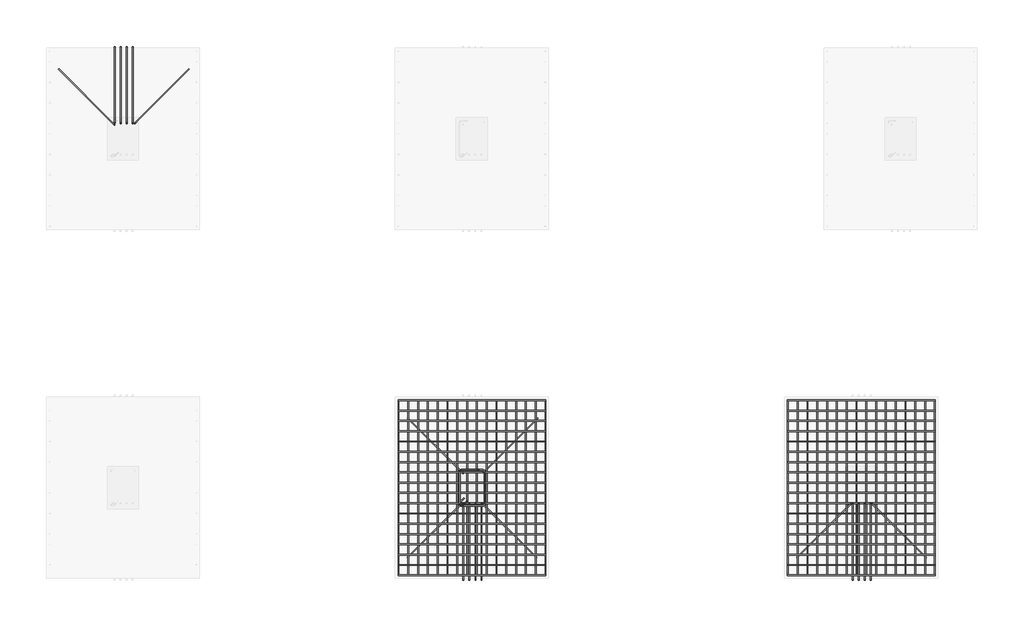
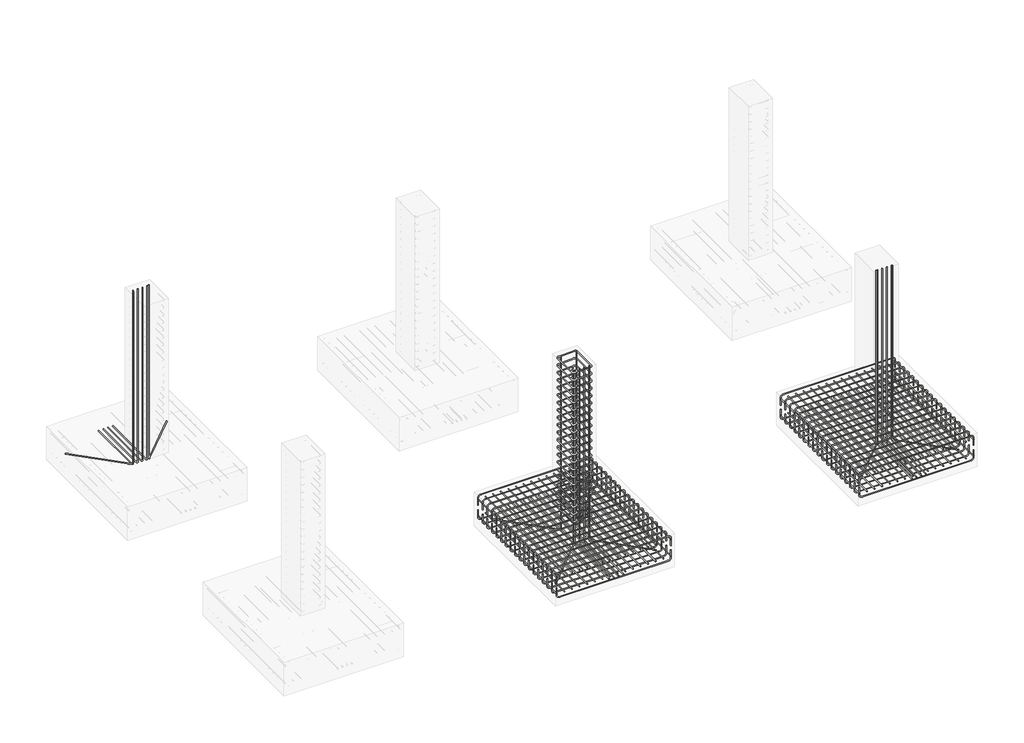
# One storey, part 11 of 33: 20 reinforcing bars.
"""IFC4 building model written with IfcOpenShell, lengths in millimetres."""

from ifc_helpers import new_model, si_unit, point, frame, origin, place, context, project, spatial, polyline, circle_curve, trimmed, segment, composite_curve, source, transform, mapped, element, save
from ifc_brep_helpers import swept_disk

model = new_model("IFC4")

# Units and contexts
model_context = context("Model", 3, world=origin())
ifc_project = project(units=[si_unit("LENGTHUNIT", "METRE", prefix="MILLI")], contexts=[model_context])

# Site, building, storey
site = spatial("IfcSite", under=ifc_project)
building = spatial("IfcBuilding", under=site)
storey = spatial("IfcBuildingStorey", under=building, Elevation=-3000.0)

# Reinforcing bars
placement = place(None, origin())
reinforcing_bar_shape = source(origin(), model_context, "Body", "SolidModel", [
    swept_disk(composite_curve([segment(polyline([(24889.0333949, -7044.0608134, -3240.0), (24889.0333949, -7044.0608134, -3092.7)]), True, "CONTINUOUS"), segment(trimmed(circle_curve(frame((24935.3833949, -7044.0608134, -3092.7), z_axis=(0.0, 1.0, 0.0), x_axis=(-46.349999999998545, 0.0, 0.0)), 46.35), [point((24889.0333949, -7044.0608134, -3092.7))], [point((24935.3833949, -7044.0608134, -3046.35))], True, "CARTESIAN"), True, "CONTINUOUS"), segment(polyline([(24935.3833949, -7044.0608134, -3046.35), (26949.9833949, -7044.0608134, -3046.35)]), True, "CONTINUOUS"), segment(trimmed(circle_curve(frame((26949.9833949, -7044.0608134, -3092.7), z_axis=(0.0, 1.0, 0.0), x_axis=(0.0, 0.0, 46.34999999999991)), 46.35), [point((26949.9833949, -7044.0608134, -3046.35))], [point((26996.3333949, -7044.0608134, -3092.7))], True, "CARTESIAN"), True, "CONTINUOUS"), segment(polyline([(26996.3333949, -7044.0608134, -3092.7), (26996.3333949, -7044.0608134, -3240.0)]), True, "CONTINUOUS")], self_intersect=False), 6.35),
])
element("IfcReinforcingBar", 1, at=placement, inside=storey, context=model_context, shape_type="MappedRepresentation", body=[
    mapped(reinforcing_bar_shape, transform((0.0, 0.0, 0.0), x_axis=(1.0, 0.0, 0.0), y_axis=(0.0, 1.0, 0.0), z_axis=(0.0, 0.0, 1.0))),
    mapped(reinforcing_bar_shape, transform((0.0, -147.4882353, 0.0), x_axis=(1.0, 0.0, 0.0), y_axis=(0.0, 1.0, 0.0), z_axis=(0.0, 0.0, 1.0))),
    mapped(reinforcing_bar_shape, transform((0.0, -294.9764706, 0.0), x_axis=(1.0, 0.0, 0.0), y_axis=(0.0, 1.0, 0.0), z_axis=(0.0, 0.0, 1.0))),
    mapped(reinforcing_bar_shape, transform((0.0, -442.4647059, 0.0), x_axis=(1.0, 0.0, 0.0), y_axis=(0.0, 1.0, 0.0), z_axis=(0.0, 0.0, 1.0))),
    mapped(reinforcing_bar_shape, transform((0.0, -589.9529412, 0.0), x_axis=(1.0, 0.0, 0.0), y_axis=(0.0, 1.0, 0.0), z_axis=(0.0, 0.0, 1.0))),
    mapped(reinforcing_bar_shape, transform((0.0, -737.4411765, 0.0), x_axis=(1.0, 0.0, 0.0), y_axis=(0.0, 1.0, 0.0), z_axis=(0.0, 0.0, 1.0))),
    mapped(reinforcing_bar_shape, transform((0.0, -884.9294118, 0.0), x_axis=(1.0, 0.0, 0.0), y_axis=(0.0, 1.0, 0.0), z_axis=(0.0, 0.0, 1.0))),
    mapped(reinforcing_bar_shape, transform((0.0, -1032.4176471, 0.0), x_axis=(1.0, 0.0, 0.0), y_axis=(0.0, 1.0, 0.0), z_axis=(0.0, 0.0, 1.0))),
    mapped(reinforcing_bar_shape, transform((0.0, -1179.9058824, 0.0), x_axis=(1.0, 0.0, 0.0), y_axis=(0.0, 1.0, 0.0), z_axis=(0.0, 0.0, 1.0))),
    mapped(reinforcing_bar_shape, transform((0.0, -1327.3941176, 0.0), x_axis=(1.0, 0.0, 0.0), y_axis=(0.0, 1.0, 0.0), z_axis=(0.0, 0.0, 1.0))),
    mapped(reinforcing_bar_shape, transform((0.0, -1474.8823529, 0.0), x_axis=(1.0, 0.0, 0.0), y_axis=(0.0, 1.0, 0.0), z_axis=(0.0, 0.0, 1.0))),
    mapped(reinforcing_bar_shape, transform((0.0, -1622.3705882, 0.0), x_axis=(1.0, 0.0, 0.0), y_axis=(0.0, 1.0, 0.0), z_axis=(0.0, 0.0, 1.0))),
    mapped(reinforcing_bar_shape, transform((0.0, -1769.8588235, 0.0), x_axis=(1.0, 0.0, 0.0), y_axis=(0.0, 1.0, 0.0), z_axis=(0.0, 0.0, 1.0))),
    mapped(reinforcing_bar_shape, transform((0.0, -1917.3470588, 0.0), x_axis=(1.0, 0.0, 0.0), y_axis=(0.0, 1.0, 0.0), z_axis=(0.0, 0.0, 1.0))),
    mapped(reinforcing_bar_shape, transform((0.0, -2064.8352941, 0.0), x_axis=(1.0, 0.0, 0.0), y_axis=(0.0, 1.0, 0.0), z_axis=(0.0, 0.0, 1.0))),
    mapped(reinforcing_bar_shape, transform((0.0, -2212.3235294, 0.0), x_axis=(1.0, 0.0, 0.0), y_axis=(0.0, 1.0, 0.0), z_axis=(0.0, 0.0, 1.0))),
    mapped(reinforcing_bar_shape, transform((0.0, -2359.8117647, 0.0), x_axis=(1.0, 0.0, 0.0), y_axis=(0.0, 1.0, 0.0), z_axis=(0.0, 0.0, 1.0))),
    mapped(reinforcing_bar_shape, transform((0.0, -2507.3, 0.0), x_axis=(1.0, 0.0, 0.0), y_axis=(0.0, 1.0, 0.0), z_axis=(0.0, 0.0, 1.0))),
])
reinforcing_bar_2_shape = source(origin(), model_context, "Body", "SolidModel", [
    swept_disk(composite_curve([segment(polyline([(26996.3333949, -7044.0608134, -3330.080452), (26996.3333949, -7044.0608134, -3477.380452)]), True, "CONTINUOUS"), segment(trimmed(circle_curve(frame((26949.9833949, -7044.0608134, -3477.380452), z_axis=(0.0, 1.0, 0.0), x_axis=(46.35000000000218, 0.0, 0.0)), 46.35), [point((26996.3333949, -7044.0608134, -3477.380452))], [point((26949.9833949, -7044.0608134, -3523.730452))], True, "CARTESIAN"), True, "CONTINUOUS"), segment(polyline([(26949.9833949, -7044.0608134, -3523.730452), (24935.3833949, -7044.0608134, -3523.730452)]), True, "CONTINUOUS"), segment(trimmed(circle_curve(frame((24935.3833949, -7044.0608134, -3477.380452), z_axis=(0.0, 1.0, 0.0), x_axis=(0.0, 0.0, -46.34999999999991)), 46.35), [point((24935.3833949, -7044.0608134, -3523.730452))], [point((24889.0333949, -7044.0608134, -3477.380452))], True, "CARTESIAN"), True, "CONTINUOUS"), segment(polyline([(24889.0333949, -7044.0608134, -3477.380452), (24889.0333949, -7044.0608134, -3330.080452)]), True, "CONTINUOUS")], self_intersect=False), 6.35),
])
element("IfcReinforcingBar", 2, at=placement, inside=storey, context=model_context, shape_type="MappedRepresentation", body=[
    mapped(reinforcing_bar_2_shape, transform((0.0, 0.0, 0.0), x_axis=(1.0, 0.0, 0.0), y_axis=(0.0, 1.0, 0.0), z_axis=(0.0, 0.0, 1.0))),
    mapped(reinforcing_bar_2_shape, transform((0.0, -147.4882353, 0.0), x_axis=(1.0, 0.0, 0.0), y_axis=(0.0, 1.0, 0.0), z_axis=(0.0, 0.0, 1.0))),
    mapped(reinforcing_bar_2_shape, transform((0.0, -294.9764706, 0.0), x_axis=(1.0, 0.0, 0.0), y_axis=(0.0, 1.0, 0.0), z_axis=(0.0, 0.0, 1.0))),
    mapped(reinforcing_bar_2_shape, transform((0.0, -442.4647059, 0.0), x_axis=(1.0, 0.0, 0.0), y_axis=(0.0, 1.0, 0.0), z_axis=(0.0, 0.0, 1.0))),
    mapped(reinforcing_bar_2_shape, transform((0.0, -589.9529412, 0.0), x_axis=(1.0, 0.0, 0.0), y_axis=(0.0, 1.0, 0.0), z_axis=(0.0, 0.0, 1.0))),
    mapped(reinforcing_bar_2_shape, transform((0.0, -737.4411765, 0.0), x_axis=(1.0, 0.0, 0.0), y_axis=(0.0, 1.0, 0.0), z_axis=(0.0, 0.0, 1.0))),
    mapped(reinforcing_bar_2_shape, transform((0.0, -884.9294118, 0.0), x_axis=(1.0, 0.0, 0.0), y_axis=(0.0, 1.0, 0.0), z_axis=(0.0, 0.0, 1.0))),
    mapped(reinforcing_bar_2_shape, transform((0.0, -1032.4176471, 0.0), x_axis=(1.0, 0.0, 0.0), y_axis=(0.0, 1.0, 0.0), z_axis=(0.0, 0.0, 1.0))),
    mapped(reinforcing_bar_2_shape, transform((0.0, -1179.9058824, 0.0), x_axis=(1.0, 0.0, 0.0), y_axis=(0.0, 1.0, 0.0), z_axis=(0.0, 0.0, 1.0))),
    mapped(reinforcing_bar_2_shape, transform((0.0, -1327.3941176, 0.0), x_axis=(1.0, 0.0, 0.0), y_axis=(0.0, 1.0, 0.0), z_axis=(0.0, 0.0, 1.0))),
    mapped(reinforcing_bar_2_shape, transform((0.0, -1474.8823529, 0.0), x_axis=(1.0, 0.0, 0.0), y_axis=(0.0, 1.0, 0.0), z_axis=(0.0, 0.0, 1.0))),
    mapped(reinforcing_bar_2_shape, transform((0.0, -1622.3705882, 0.0), x_axis=(1.0, 0.0, 0.0), y_axis=(0.0, 1.0, 0.0), z_axis=(0.0, 0.0, 1.0))),
    mapped(reinforcing_bar_2_shape, transform((0.0, -1769.8588235, 0.0), x_axis=(1.0, 0.0, 0.0), y_axis=(0.0, 1.0, 0.0), z_axis=(0.0, 0.0, 1.0))),
    mapped(reinforcing_bar_2_shape, transform((0.0, -1917.3470588, 0.0), x_axis=(1.0, 0.0, 0.0), y_axis=(0.0, 1.0, 0.0), z_axis=(0.0, 0.0, 1.0))),
    mapped(reinforcing_bar_2_shape, transform((0.0, -2064.8352941, 0.0), x_axis=(1.0, 0.0, 0.0), y_axis=(0.0, 1.0, 0.0), z_axis=(0.0, 0.0, 1.0))),
    mapped(reinforcing_bar_2_shape, transform((0.0, -2212.3235294, 0.0), x_axis=(1.0, 0.0, 0.0), y_axis=(0.0, 1.0, 0.0), z_axis=(0.0, 0.0, 1.0))),
    mapped(reinforcing_bar_2_shape, transform((0.0, -2359.8117647, 0.0), x_axis=(1.0, 0.0, 0.0), y_axis=(0.0, 1.0, 0.0), z_axis=(0.0, 0.0, 1.0))),
    mapped(reinforcing_bar_2_shape, transform((0.0, -2507.3, 0.0), x_axis=(1.0, 0.0, 0.0), y_axis=(0.0, 1.0, 0.0), z_axis=(0.0, 0.0, 1.0))),
])
reinforcing_bar_3_shape = source(origin(), model_context, "Body", "SolidModel", [
    swept_disk(composite_curve([segment(polyline([(26996.3333949, -9557.7108134, -3447.8614173), (26996.3333949, -7037.7108134, -3447.8614173)]), True, "CONTINUOUS")], self_intersect=False), 6.35),
])
element("IfcReinforcingBar", 3, at=placement, inside=storey, context=model_context, shape_type="MappedRepresentation", body=[
    mapped(reinforcing_bar_3_shape, transform((0.0, 0.0, 0.0), x_axis=(1.0, 0.0, 0.0), y_axis=(0.0, 1.0, 0.0), z_axis=(0.0, 0.0, 1.0))),
    mapped(reinforcing_bar_3_shape, transform((-140.4866667, 0.0, 0.0), x_axis=(1.0, 0.0, 0.0), y_axis=(0.0, 1.0, 0.0), z_axis=(0.0, 0.0, 1.0))),
    mapped(reinforcing_bar_3_shape, transform((-280.9733333, 0.0, 0.0), x_axis=(1.0, 0.0, 0.0), y_axis=(0.0, 1.0, 0.0), z_axis=(0.0, 0.0, 1.0))),
    mapped(reinforcing_bar_3_shape, transform((-421.46, 0.0, 0.0), x_axis=(1.0, 0.0, 0.0), y_axis=(0.0, 1.0, 0.0), z_axis=(0.0, 0.0, 1.0))),
    mapped(reinforcing_bar_3_shape, transform((-561.9466667, 0.0, 0.0), x_axis=(1.0, 0.0, 0.0), y_axis=(0.0, 1.0, 0.0), z_axis=(0.0, 0.0, 1.0))),
    mapped(reinforcing_bar_3_shape, transform((-702.4333333, 0.0, 0.0), x_axis=(1.0, 0.0, 0.0), y_axis=(0.0, 1.0, 0.0), z_axis=(0.0, 0.0, 1.0))),
    mapped(reinforcing_bar_3_shape, transform((-842.92, 0.0, 0.0), x_axis=(1.0, 0.0, 0.0), y_axis=(0.0, 1.0, 0.0), z_axis=(0.0, 0.0, 1.0))),
    mapped(reinforcing_bar_3_shape, transform((-983.4066667, 0.0, 0.0), x_axis=(1.0, 0.0, 0.0), y_axis=(0.0, 1.0, 0.0), z_axis=(0.0, 0.0, 1.0))),
    mapped(reinforcing_bar_3_shape, transform((-1123.8933333, 0.0, 0.0), x_axis=(1.0, 0.0, 0.0), y_axis=(0.0, 1.0, 0.0), z_axis=(0.0, 0.0, 1.0))),
    mapped(reinforcing_bar_3_shape, transform((-1264.38, 0.0, 0.0), x_axis=(1.0, 0.0, 0.0), y_axis=(0.0, 1.0, 0.0), z_axis=(0.0, 0.0, 1.0))),
    mapped(reinforcing_bar_3_shape, transform((-1404.8666667, 0.0, 0.0), x_axis=(1.0, 0.0, 0.0), y_axis=(0.0, 1.0, 0.0), z_axis=(0.0, 0.0, 1.0))),
    mapped(reinforcing_bar_3_shape, transform((-1545.3533333, 0.0, 0.0), x_axis=(1.0, 0.0, 0.0), y_axis=(0.0, 1.0, 0.0), z_axis=(0.0, 0.0, 1.0))),
    mapped(reinforcing_bar_3_shape, transform((-1685.84, 0.0, 0.0), x_axis=(1.0, 0.0, 0.0), y_axis=(0.0, 1.0, 0.0), z_axis=(0.0, 0.0, 1.0))),
    mapped(reinforcing_bar_3_shape, transform((-1826.3266667, 0.0, 0.0), x_axis=(1.0, 0.0, 0.0), y_axis=(0.0, 1.0, 0.0), z_axis=(0.0, 0.0, 1.0))),
    mapped(reinforcing_bar_3_shape, transform((-1966.8133333, 0.0, 0.0), x_axis=(1.0, 0.0, 0.0), y_axis=(0.0, 1.0, 0.0), z_axis=(0.0, 0.0, 1.0))),
    mapped(reinforcing_bar_3_shape, transform((-2107.3, 0.0, 0.0), x_axis=(1.0, 0.0, 0.0), y_axis=(0.0, 1.0, 0.0), z_axis=(0.0, 0.0, 1.0))),
])
reinforcing_bar_4_shape = source(origin(), model_context, "Body", "SolidModel", [
    swept_disk(composite_curve([segment(polyline([(24889.0333949, -9557.7108134, -3122.7084113), (24889.0333949, -7037.7108134, -3122.7084113)]), True, "CONTINUOUS")], self_intersect=False), 6.35),
])
element("IfcReinforcingBar", 4, at=placement, inside=storey, context=model_context, shape_type="MappedRepresentation", body=[
    mapped(reinforcing_bar_4_shape, transform((0.0, 0.0, 0.0), x_axis=(1.0, 0.0, 0.0), y_axis=(0.0, 1.0, 0.0), z_axis=(0.0, 0.0, 1.0))),
    mapped(reinforcing_bar_4_shape, transform((140.4866667, 0.0, 0.0), x_axis=(1.0, 0.0, 0.0), y_axis=(0.0, 1.0, 0.0), z_axis=(0.0, 0.0, 1.0))),
    mapped(reinforcing_bar_4_shape, transform((280.9733333, 0.0, 0.0), x_axis=(1.0, 0.0, 0.0), y_axis=(0.0, 1.0, 0.0), z_axis=(0.0, 0.0, 1.0))),
    mapped(reinforcing_bar_4_shape, transform((421.46, 0.0, 0.0), x_axis=(1.0, 0.0, 0.0), y_axis=(0.0, 1.0, 0.0), z_axis=(0.0, 0.0, 1.0))),
    mapped(reinforcing_bar_4_shape, transform((561.9466667, 0.0, 0.0), x_axis=(1.0, 0.0, 0.0), y_axis=(0.0, 1.0, 0.0), z_axis=(0.0, 0.0, 1.0))),
    mapped(reinforcing_bar_4_shape, transform((702.4333333, 0.0, 0.0), x_axis=(1.0, 0.0, 0.0), y_axis=(0.0, 1.0, 0.0), z_axis=(0.0, 0.0, 1.0))),
    mapped(reinforcing_bar_4_shape, transform((842.92, 0.0, 0.0), x_axis=(1.0, 0.0, 0.0), y_axis=(0.0, 1.0, 0.0), z_axis=(0.0, 0.0, 1.0))),
    mapped(reinforcing_bar_4_shape, transform((983.4066667, 0.0, 0.0), x_axis=(1.0, 0.0, 0.0), y_axis=(0.0, 1.0, 0.0), z_axis=(0.0, 0.0, 1.0))),
    mapped(reinforcing_bar_4_shape, transform((1123.8933333, 0.0, 0.0), x_axis=(1.0, 0.0, 0.0), y_axis=(0.0, 1.0, 0.0), z_axis=(0.0, 0.0, 1.0))),
    mapped(reinforcing_bar_4_shape, transform((1264.38, 0.0, 0.0), x_axis=(1.0, 0.0, 0.0), y_axis=(0.0, 1.0, 0.0), z_axis=(0.0, 0.0, 1.0))),
    mapped(reinforcing_bar_4_shape, transform((1404.8666667, 0.0, 0.0), x_axis=(1.0, 0.0, 0.0), y_axis=(0.0, 1.0, 0.0), z_axis=(0.0, 0.0, 1.0))),
    mapped(reinforcing_bar_4_shape, transform((1545.3533333, 0.0, 0.0), x_axis=(1.0, 0.0, 0.0), y_axis=(0.0, 1.0, 0.0), z_axis=(0.0, 0.0, 1.0))),
    mapped(reinforcing_bar_4_shape, transform((1685.84, 0.0, 0.0), x_axis=(1.0, 0.0, 0.0), y_axis=(0.0, 1.0, 0.0), z_axis=(0.0, 0.0, 1.0))),
    mapped(reinforcing_bar_4_shape, transform((1826.3266667, 0.0, 0.0), x_axis=(1.0, 0.0, 0.0), y_axis=(0.0, 1.0, 0.0), z_axis=(0.0, 0.0, 1.0))),
    mapped(reinforcing_bar_4_shape, transform((1966.8133333, 0.0, 0.0), x_axis=(1.0, 0.0, 0.0), y_axis=(0.0, 1.0, 0.0), z_axis=(0.0, 0.0, 1.0))),
    mapped(reinforcing_bar_4_shape, transform((2107.3, 0.0, 0.0), x_axis=(1.0, 0.0, 0.0), y_axis=(0.0, 1.0, 0.0), z_axis=(0.0, 0.0, 1.0))),
])
reinforcing_bar_5_shape = source(origin(), model_context, "Body", "SolidModel", [
    swept_disk(composite_curve([segment(polyline([(19306.5357258, -7044.0608134, -3240.0), (19306.5357258, -7044.0608134, -3092.7)]), True, "CONTINUOUS"), segment(trimmed(circle_curve(frame((19352.8857258, -7044.0608134, -3092.7), z_axis=(0.0, 1.0, 0.0), x_axis=(-46.349999999998545, 0.0, 0.0)), 46.35), [point((19306.5357258, -7044.0608134, -3092.7))], [point((19352.8857258, -7044.0608134, -3046.35))], True, "CARTESIAN"), True, "CONTINUOUS"), segment(polyline([(19352.8857258, -7044.0608134, -3046.35), (21367.4857258, -7044.0608134, -3046.35)]), True, "CONTINUOUS"), segment(trimmed(circle_curve(frame((21367.4857258, -7044.0608134, -3092.7), z_axis=(0.0, 1.0, 0.0), x_axis=(0.0, 0.0, 46.34999999999991)), 46.35), [point((21367.4857258, -7044.0608134, -3046.35))], [point((21413.8357258, -7044.0608134, -3092.7))], True, "CARTESIAN"), True, "CONTINUOUS"), segment(polyline([(21413.8357258, -7044.0608134, -3092.7), (21413.8357258, -7044.0608134, -3240.0)]), True, "CONTINUOUS")], self_intersect=False), 6.35),
])
element("IfcReinforcingBar", 5, at=placement, inside=storey, context=model_context, shape_type="MappedRepresentation", body=[
    mapped(reinforcing_bar_5_shape, transform((0.0, 0.0, 0.0), x_axis=(1.0, 0.0, 0.0), y_axis=(0.0, 1.0, 0.0), z_axis=(0.0, 0.0, 1.0))),
    mapped(reinforcing_bar_5_shape, transform((0.0, -147.4882353, 0.0), x_axis=(1.0, 0.0, 0.0), y_axis=(0.0, 1.0, 0.0), z_axis=(0.0, 0.0, 1.0))),
    mapped(reinforcing_bar_5_shape, transform((0.0, -294.9764706, 0.0), x_axis=(1.0, 0.0, 0.0), y_axis=(0.0, 1.0, 0.0), z_axis=(0.0, 0.0, 1.0))),
    mapped(reinforcing_bar_5_shape, transform((0.0, -442.4647059, 0.0), x_axis=(1.0, 0.0, 0.0), y_axis=(0.0, 1.0, 0.0), z_axis=(0.0, 0.0, 1.0))),
    mapped(reinforcing_bar_5_shape, transform((0.0, -589.9529412, 0.0), x_axis=(1.0, 0.0, 0.0), y_axis=(0.0, 1.0, 0.0), z_axis=(0.0, 0.0, 1.0))),
    mapped(reinforcing_bar_5_shape, transform((0.0, -737.4411765, 0.0), x_axis=(1.0, 0.0, 0.0), y_axis=(0.0, 1.0, 0.0), z_axis=(0.0, 0.0, 1.0))),
    mapped(reinforcing_bar_5_shape, transform((0.0, -884.9294118, 0.0), x_axis=(1.0, 0.0, 0.0), y_axis=(0.0, 1.0, 0.0), z_axis=(0.0, 0.0, 1.0))),
    mapped(reinforcing_bar_5_shape, transform((0.0, -1032.4176471, 0.0), x_axis=(1.0, 0.0, 0.0), y_axis=(0.0, 1.0, 0.0), z_axis=(0.0, 0.0, 1.0))),
    mapped(reinforcing_bar_5_shape, transform((0.0, -1179.9058824, 0.0), x_axis=(1.0, 0.0, 0.0), y_axis=(0.0, 1.0, 0.0), z_axis=(0.0, 0.0, 1.0))),
    mapped(reinforcing_bar_5_shape, transform((0.0, -1327.3941176, 0.0), x_axis=(1.0, 0.0, 0.0), y_axis=(0.0, 1.0, 0.0), z_axis=(0.0, 0.0, 1.0))),
    mapped(reinforcing_bar_5_shape, transform((0.0, -1474.8823529, 0.0), x_axis=(1.0, 0.0, 0.0), y_axis=(0.0, 1.0, 0.0), z_axis=(0.0, 0.0, 1.0))),
    mapped(reinforcing_bar_5_shape, transform((0.0, -1622.3705882, 0.0), x_axis=(1.0, 0.0, 0.0), y_axis=(0.0, 1.0, 0.0), z_axis=(0.0, 0.0, 1.0))),
    mapped(reinforcing_bar_5_shape, transform((0.0, -1769.8588235, 0.0), x_axis=(1.0, 0.0, 0.0), y_axis=(0.0, 1.0, 0.0), z_axis=(0.0, 0.0, 1.0))),
    mapped(reinforcing_bar_5_shape, transform((0.0, -1917.3470588, 0.0), x_axis=(1.0, 0.0, 0.0), y_axis=(0.0, 1.0, 0.0), z_axis=(0.0, 0.0, 1.0))),
    mapped(reinforcing_bar_5_shape, transform((0.0, -2064.8352941, 0.0), x_axis=(1.0, 0.0, 0.0), y_axis=(0.0, 1.0, 0.0), z_axis=(0.0, 0.0, 1.0))),
    mapped(reinforcing_bar_5_shape, transform((0.0, -2212.3235294, 0.0), x_axis=(1.0, 0.0, 0.0), y_axis=(0.0, 1.0, 0.0), z_axis=(0.0, 0.0, 1.0))),
    mapped(reinforcing_bar_5_shape, transform((0.0, -2359.8117647, 0.0), x_axis=(1.0, 0.0, 0.0), y_axis=(0.0, 1.0, 0.0), z_axis=(0.0, 0.0, 1.0))),
    mapped(reinforcing_bar_5_shape, transform((0.0, -2507.3, 0.0), x_axis=(1.0, 0.0, 0.0), y_axis=(0.0, 1.0, 0.0), z_axis=(0.0, 0.0, 1.0))),
])
reinforcing_bar_6_shape = source(origin(), model_context, "Body", "SolidModel", [
    swept_disk(composite_curve([segment(polyline([(21413.8357258, -7044.0608134, -3330.080452), (21413.8357258, -7044.0608134, -3477.380452)]), True, "CONTINUOUS"), segment(trimmed(circle_curve(frame((21367.4857258, -7044.0608134, -3477.380452), z_axis=(0.0, 1.0, 0.0), x_axis=(46.349999999998545, 0.0, 0.0)), 46.35), [point((21413.8357258, -7044.0608134, -3477.380452))], [point((21367.4857258, -7044.0608134, -3523.730452))], True, "CARTESIAN"), True, "CONTINUOUS"), segment(polyline([(21367.4857258, -7044.0608134, -3523.730452), (19352.8857258, -7044.0608134, -3523.730452)]), True, "CONTINUOUS"), segment(trimmed(circle_curve(frame((19352.8857258, -7044.0608134, -3477.380452), z_axis=(0.0, 1.0, 0.0), x_axis=(0.0, 0.0, -46.34999999999991)), 46.35), [point((19352.8857258, -7044.0608134, -3523.730452))], [point((19306.5357258, -7044.0608134, -3477.380452))], True, "CARTESIAN"), True, "CONTINUOUS"), segment(polyline([(19306.5357258, -7044.0608134, -3477.380452), (19306.5357258, -7044.0608134, -3330.080452)]), True, "CONTINUOUS")], self_intersect=False), 6.35),
])
element("IfcReinforcingBar", 6, at=placement, inside=storey, context=model_context, shape_type="MappedRepresentation", body=[
    mapped(reinforcing_bar_6_shape, transform((0.0, 0.0, 0.0), x_axis=(1.0, 0.0, 0.0), y_axis=(0.0, 1.0, 0.0), z_axis=(0.0, 0.0, 1.0))),
    mapped(reinforcing_bar_6_shape, transform((0.0, -147.4882353, 0.0), x_axis=(1.0, 0.0, 0.0), y_axis=(0.0, 1.0, 0.0), z_axis=(0.0, 0.0, 1.0))),
    mapped(reinforcing_bar_6_shape, transform((0.0, -294.9764706, 0.0), x_axis=(1.0, 0.0, 0.0), y_axis=(0.0, 1.0, 0.0), z_axis=(0.0, 0.0, 1.0))),
    mapped(reinforcing_bar_6_shape, transform((0.0, -442.4647059, 0.0), x_axis=(1.0, 0.0, 0.0), y_axis=(0.0, 1.0, 0.0), z_axis=(0.0, 0.0, 1.0))),
    mapped(reinforcing_bar_6_shape, transform((0.0, -589.9529412, 0.0), x_axis=(1.0, 0.0, 0.0), y_axis=(0.0, 1.0, 0.0), z_axis=(0.0, 0.0, 1.0))),
    mapped(reinforcing_bar_6_shape, transform((0.0, -737.4411765, 0.0), x_axis=(1.0, 0.0, 0.0), y_axis=(0.0, 1.0, 0.0), z_axis=(0.0, 0.0, 1.0))),
    mapped(reinforcing_bar_6_shape, transform((0.0, -884.9294118, 0.0), x_axis=(1.0, 0.0, 0.0), y_axis=(0.0, 1.0, 0.0), z_axis=(0.0, 0.0, 1.0))),
    mapped(reinforcing_bar_6_shape, transform((0.0, -1032.4176471, 0.0), x_axis=(1.0, 0.0, 0.0), y_axis=(0.0, 1.0, 0.0), z_axis=(0.0, 0.0, 1.0))),
    mapped(reinforcing_bar_6_shape, transform((0.0, -1179.9058824, 0.0), x_axis=(1.0, 0.0, 0.0), y_axis=(0.0, 1.0, 0.0), z_axis=(0.0, 0.0, 1.0))),
    mapped(reinforcing_bar_6_shape, transform((0.0, -1327.3941176, 0.0), x_axis=(1.0, 0.0, 0.0), y_axis=(0.0, 1.0, 0.0), z_axis=(0.0, 0.0, 1.0))),
    mapped(reinforcing_bar_6_shape, transform((0.0, -1474.8823529, 0.0), x_axis=(1.0, 0.0, 0.0), y_axis=(0.0, 1.0, 0.0), z_axis=(0.0, 0.0, 1.0))),
    mapped(reinforcing_bar_6_shape, transform((0.0, -1622.3705882, 0.0), x_axis=(1.0, 0.0, 0.0), y_axis=(0.0, 1.0, 0.0), z_axis=(0.0, 0.0, 1.0))),
    mapped(reinforcing_bar_6_shape, transform((0.0, -1769.8588235, 0.0), x_axis=(1.0, 0.0, 0.0), y_axis=(0.0, 1.0, 0.0), z_axis=(0.0, 0.0, 1.0))),
    mapped(reinforcing_bar_6_shape, transform((0.0, -1917.3470588, 0.0), x_axis=(1.0, 0.0, 0.0), y_axis=(0.0, 1.0, 0.0), z_axis=(0.0, 0.0, 1.0))),
    mapped(reinforcing_bar_6_shape, transform((0.0, -2064.8352941, 0.0), x_axis=(1.0, 0.0, 0.0), y_axis=(0.0, 1.0, 0.0), z_axis=(0.0, 0.0, 1.0))),
    mapped(reinforcing_bar_6_shape, transform((0.0, -2212.3235294, 0.0), x_axis=(1.0, 0.0, 0.0), y_axis=(0.0, 1.0, 0.0), z_axis=(0.0, 0.0, 1.0))),
    mapped(reinforcing_bar_6_shape, transform((0.0, -2359.8117647, 0.0), x_axis=(1.0, 0.0, 0.0), y_axis=(0.0, 1.0, 0.0), z_axis=(0.0, 0.0, 1.0))),
    mapped(reinforcing_bar_6_shape, transform((0.0, -2507.3, 0.0), x_axis=(1.0, 0.0, 0.0), y_axis=(0.0, 1.0, 0.0), z_axis=(0.0, 0.0, 1.0))),
])
reinforcing_bar_7_shape = source(origin(), model_context, "Body", "SolidModel", [
    swept_disk(composite_curve([segment(polyline([(21413.8357258, -9557.7108134, -3447.8614173), (21413.8357258, -7037.7108134, -3447.8614173)]), True, "CONTINUOUS")], self_intersect=False), 6.35),
])
element("IfcReinforcingBar", 7, at=placement, inside=storey, context=model_context, shape_type="MappedRepresentation", body=[
    mapped(reinforcing_bar_7_shape, transform((0.0, 0.0, 0.0), x_axis=(1.0, 0.0, 0.0), y_axis=(0.0, 1.0, 0.0), z_axis=(0.0, 0.0, 1.0))),
    mapped(reinforcing_bar_7_shape, transform((-140.4866667, 0.0, 0.0), x_axis=(1.0, 0.0, 0.0), y_axis=(0.0, 1.0, 0.0), z_axis=(0.0, 0.0, 1.0))),
    mapped(reinforcing_bar_7_shape, transform((-280.9733333, 0.0, 0.0), x_axis=(1.0, 0.0, 0.0), y_axis=(0.0, 1.0, 0.0), z_axis=(0.0, 0.0, 1.0))),
    mapped(reinforcing_bar_7_shape, transform((-421.46, 0.0, 0.0), x_axis=(1.0, 0.0, 0.0), y_axis=(0.0, 1.0, 0.0), z_axis=(0.0, 0.0, 1.0))),
    mapped(reinforcing_bar_7_shape, transform((-561.9466667, 0.0, 0.0), x_axis=(1.0, 0.0, 0.0), y_axis=(0.0, 1.0, 0.0), z_axis=(0.0, 0.0, 1.0))),
    mapped(reinforcing_bar_7_shape, transform((-702.4333333, 0.0, 0.0), x_axis=(1.0, 0.0, 0.0), y_axis=(0.0, 1.0, 0.0), z_axis=(0.0, 0.0, 1.0))),
    mapped(reinforcing_bar_7_shape, transform((-842.92, 0.0, 0.0), x_axis=(1.0, 0.0, 0.0), y_axis=(0.0, 1.0, 0.0), z_axis=(0.0, 0.0, 1.0))),
    mapped(reinforcing_bar_7_shape, transform((-983.4066667, 0.0, 0.0), x_axis=(1.0, 0.0, 0.0), y_axis=(0.0, 1.0, 0.0), z_axis=(0.0, 0.0, 1.0))),
    mapped(reinforcing_bar_7_shape, transform((-1123.8933333, 0.0, 0.0), x_axis=(1.0, 0.0, 0.0), y_axis=(0.0, 1.0, 0.0), z_axis=(0.0, 0.0, 1.0))),
    mapped(reinforcing_bar_7_shape, transform((-1264.38, 0.0, 0.0), x_axis=(1.0, 0.0, 0.0), y_axis=(0.0, 1.0, 0.0), z_axis=(0.0, 0.0, 1.0))),
    mapped(reinforcing_bar_7_shape, transform((-1404.8666667, 0.0, 0.0), x_axis=(1.0, 0.0, 0.0), y_axis=(0.0, 1.0, 0.0), z_axis=(0.0, 0.0, 1.0))),
    mapped(reinforcing_bar_7_shape, transform((-1545.3533333, 0.0, 0.0), x_axis=(1.0, 0.0, 0.0), y_axis=(0.0, 1.0, 0.0), z_axis=(0.0, 0.0, 1.0))),
    mapped(reinforcing_bar_7_shape, transform((-1685.84, 0.0, 0.0), x_axis=(1.0, 0.0, 0.0), y_axis=(0.0, 1.0, 0.0), z_axis=(0.0, 0.0, 1.0))),
    mapped(reinforcing_bar_7_shape, transform((-1826.3266667, 0.0, 0.0), x_axis=(1.0, 0.0, 0.0), y_axis=(0.0, 1.0, 0.0), z_axis=(0.0, 0.0, 1.0))),
    mapped(reinforcing_bar_7_shape, transform((-1966.8133333, 0.0, 0.0), x_axis=(1.0, 0.0, 0.0), y_axis=(0.0, 1.0, 0.0), z_axis=(0.0, 0.0, 1.0))),
    mapped(reinforcing_bar_7_shape, transform((-2107.3, 0.0, 0.0), x_axis=(1.0, 0.0, 0.0), y_axis=(0.0, 1.0, 0.0), z_axis=(0.0, 0.0, 1.0))),
])
reinforcing_bar_8_shape = source(origin(), model_context, "Body", "SolidModel", [
    swept_disk(composite_curve([segment(polyline([(19306.5357258, -9557.7108134, -3122.7084113), (19306.5357258, -7037.7108134, -3122.7084113)]), True, "CONTINUOUS")], self_intersect=False), 6.35),
])
element("IfcReinforcingBar", 8, at=placement, inside=storey, context=model_context, shape_type="MappedRepresentation", body=[
    mapped(reinforcing_bar_8_shape, transform((0.0, 0.0, 0.0), x_axis=(1.0, 0.0, 0.0), y_axis=(0.0, 1.0, 0.0), z_axis=(0.0, 0.0, 1.0))),
    mapped(reinforcing_bar_8_shape, transform((140.4866667, 0.0, 0.0), x_axis=(1.0, 0.0, 0.0), y_axis=(0.0, 1.0, 0.0), z_axis=(0.0, 0.0, 1.0))),
    mapped(reinforcing_bar_8_shape, transform((280.9733333, 0.0, 0.0), x_axis=(1.0, 0.0, 0.0), y_axis=(0.0, 1.0, 0.0), z_axis=(0.0, 0.0, 1.0))),
    mapped(reinforcing_bar_8_shape, transform((421.46, 0.0, 0.0), x_axis=(1.0, 0.0, 0.0), y_axis=(0.0, 1.0, 0.0), z_axis=(0.0, 0.0, 1.0))),
    mapped(reinforcing_bar_8_shape, transform((561.9466667, 0.0, 0.0), x_axis=(1.0, 0.0, 0.0), y_axis=(0.0, 1.0, 0.0), z_axis=(0.0, 0.0, 1.0))),
    mapped(reinforcing_bar_8_shape, transform((702.4333333, 0.0, 0.0), x_axis=(1.0, 0.0, 0.0), y_axis=(0.0, 1.0, 0.0), z_axis=(0.0, 0.0, 1.0))),
    mapped(reinforcing_bar_8_shape, transform((842.92, 0.0, 0.0), x_axis=(1.0, 0.0, 0.0), y_axis=(0.0, 1.0, 0.0), z_axis=(0.0, 0.0, 1.0))),
    mapped(reinforcing_bar_8_shape, transform((983.4066667, 0.0, 0.0), x_axis=(1.0, 0.0, 0.0), y_axis=(0.0, 1.0, 0.0), z_axis=(0.0, 0.0, 1.0))),
    mapped(reinforcing_bar_8_shape, transform((1123.8933333, 0.0, 0.0), x_axis=(1.0, 0.0, 0.0), y_axis=(0.0, 1.0, 0.0), z_axis=(0.0, 0.0, 1.0))),
    mapped(reinforcing_bar_8_shape, transform((1264.38, 0.0, 0.0), x_axis=(1.0, 0.0, 0.0), y_axis=(0.0, 1.0, 0.0), z_axis=(0.0, 0.0, 1.0))),
    mapped(reinforcing_bar_8_shape, transform((1404.8666667, 0.0, 0.0), x_axis=(1.0, 0.0, 0.0), y_axis=(0.0, 1.0, 0.0), z_axis=(0.0, 0.0, 1.0))),
    mapped(reinforcing_bar_8_shape, transform((1545.3533333, 0.0, 0.0), x_axis=(1.0, 0.0, 0.0), y_axis=(0.0, 1.0, 0.0), z_axis=(0.0, 0.0, 1.0))),
    mapped(reinforcing_bar_8_shape, transform((1685.84, 0.0, 0.0), x_axis=(1.0, 0.0, 0.0), y_axis=(0.0, 1.0, 0.0), z_axis=(0.0, 0.0, 1.0))),
    mapped(reinforcing_bar_8_shape, transform((1826.3266667, 0.0, 0.0), x_axis=(1.0, 0.0, 0.0), y_axis=(0.0, 1.0, 0.0), z_axis=(0.0, 0.0, 1.0))),
    mapped(reinforcing_bar_8_shape, transform((1966.8133333, 0.0, 0.0), x_axis=(1.0, 0.0, 0.0), y_axis=(0.0, 1.0, 0.0), z_axis=(0.0, 0.0, 1.0))),
    mapped(reinforcing_bar_8_shape, transform((2107.3, 0.0, 0.0), x_axis=(1.0, 0.0, 0.0), y_axis=(0.0, 1.0, 0.0), z_axis=(0.0, 0.0, 1.0))),
])
element("IfcReinforcingBar", 9, at=placement, inside=storey, context=model_context, shape_type="SolidModel", body=[
    swept_disk(composite_curve([segment(polyline([(15231.1024274, -3091.6857913, -40.0), (15231.1024274, -3091.6857913, -3361.434517)]), True, "CONTINUOUS"), segment(trimmed(circle_curve(frame((15198.3280281, -3058.911392, -3361.434517), z_axis=(0.7071067811865539, 0.7071067811865411, 0.0), x_axis=(32.77439929999855, -32.774399299999914, 0.0)), 46.35), [point((15231.1024274, -3091.6857913, -3361.434517))], [point((15198.3280281, -3058.911392, -3407.784517))], True, "CARTESIAN"), True, "CONTINUOUS"), segment(polyline([(15198.3280281, -3058.911392, -3407.784517), (14435.3868621, -2295.970226, -3407.784517)]), True, "CONTINUOUS")], self_intersect=False), 6.35),
])
element("IfcReinforcingBar", 10, at=placement, inside=storey, context=model_context, shape_type="SolidModel", body=[
    swept_disk(composite_curve([segment(polyline([(15525.7684217, -3073.7876853, -30.2564663), (15525.7684217, -3073.7876853, -3383.9064663)]), True, "CONTINUOUS"), segment(trimmed(circle_curve(frame((15558.542821, -3041.013286, -3383.9064663), z_axis=(0.7071067811865493, -0.7071067811865459, 0.0), x_axis=(-32.77439929999855, -32.774399299999914, 0.0)), 46.35), [point((15525.7684217, -3073.7876853, -3383.9064663))], [point((15558.542821, -3041.013286, -3430.2564663))], True, "CARTESIAN"), True, "CONTINUOUS"), segment(polyline([(15558.542821, -3041.013286, -3430.2564663), (16303.585881, -2295.970226, -3430.2564663)]), True, "CONTINUOUS")], self_intersect=False), 6.35),
])
reinforcing_bar_9_shape = source(origin(), model_context, "Body", "SolidModel", [
    swept_disk(composite_curve([segment(polyline([(15236.1158322, -3071.9278134, -40.0), (15236.1158322, -3071.9278134, -3393.65)]), True, "CONTINUOUS"), segment(trimmed(circle_curve(frame((15236.1158322, -3025.5778134, -3393.65), z_axis=(1.0, 0.0, 0.0), x_axis=(0.0, -46.34999999999991, 0.0)), 46.35), [point((15236.1158322, -3071.9278134, -3393.65))], [point((15236.1158322, -3025.5778134, -3440.0))], True, "CARTESIAN"), True, "CONTINUOUS"), segment(polyline([(15236.1158322, -3025.5778134, -3440.0), (15236.1158322, -1971.9278134, -3440.0)]), True, "CONTINUOUS")], self_intersect=False), 6.35),
])
element("IfcReinforcingBar", 11, at=placement, inside=storey, context=model_context, shape_type="MappedRepresentation", body=[
    mapped(reinforcing_bar_9_shape, transform((0.0, 0.0, 0.0), x_axis=(1.0, 0.0, 0.0), y_axis=(0.0, 1.0, 0.0), z_axis=(0.0, 0.0, 1.0))),
    mapped(reinforcing_bar_9_shape, transform((86.8979716, 0.0, 0.0), x_axis=(1.0, 0.0, 0.0), y_axis=(0.0, 1.0, 0.0), z_axis=(0.0, 0.0, 1.0))),
    mapped(reinforcing_bar_9_shape, transform((173.7959432, 0.0, 0.0), x_axis=(1.0, 0.0, 0.0), y_axis=(0.0, 1.0, 0.0), z_axis=(0.0, 0.0, 1.0))),
    mapped(reinforcing_bar_9_shape, transform((260.6939148, 0.0, 0.0), x_axis=(1.0, 0.0, 0.0), y_axis=(0.0, 1.0, 0.0), z_axis=(0.0, 0.0, 1.0))),
])
reinforcing_bar_10_shape = source(origin(), model_context, "Body", "SolidModel", [
    swept_disk(composite_curve([segment(polyline([(20246.4614911, -8446.8994528, -2953.65), (20190.7179282, -8502.6430158, -2953.65)]), True, "CONTINUOUS"), segment(trimmed(circle_curve(frame((20212.8857258, -8524.8108134, -2953.65), z_axis=(0.0, 0.0, 1.0), x_axis=(-22.167797599999176, 22.167797599999176, 0.0)), 31.35), [point((20190.7179282, -8502.6430158, -2953.65))], [point((20212.8857258, -8556.1608134, -2953.65))], True, "CARTESIAN"), True, "CONTINUOUS"), segment(polyline([(20212.8857258, -8556.1608134, -2953.65), (20507.4857258, -8556.1608134, -2953.65)]), True, "CONTINUOUS"), segment(trimmed(circle_curve(frame((20507.4857258, -8524.8108134, -2953.65), z_axis=(0.0, 0.0, 1.0), x_axis=(0.0, -31.350000000000364, 0.0)), 31.35), [point((20507.4857258, -8556.1608134, -2953.65))], [point((20538.8357258, -8524.8108134, -2953.65))], True, "CARTESIAN"), True, "CONTINUOUS"), segment(polyline([(20538.8357258, -8524.8108134, -2953.65), (20538.8357258, -8070.6108134, -2953.65)]), True, "CONTINUOUS"), segment(trimmed(circle_curve(frame((20507.5055109, -8070.6108134, -2954.7636125), z_axis=(-0.0355219283344822, 0.0, 0.9993688971583016), x_axis=(31.33021490000101, 0.0, 1.1136124999998174)), 31.35), [point((20538.8357258, -8070.6108134, -2953.65))], [point((20507.5055109, -8039.2608134, -2954.7636125))], True, "CARTESIAN"), True, "CONTINUOUS"), segment(polyline([(20507.5055109, -8039.2608134, -2954.7636125), (20212.8659407, -8039.2608134, -2965.2363875)]), True, "CONTINUOUS"), segment(trimmed(circle_curve(frame((20212.8659407, -8070.6108134, -2965.2363875), z_axis=(-0.0355219283344822, 0.0, 0.9993688971583016), x_axis=(0.0, 31.349999999999454, 0.0)), 31.35), [point((20212.8659407, -8039.2608134, -2965.2363875))], [point((20181.5357258, -8070.6108134, -2966.35))], True, "CARTESIAN"), True, "CONTINUOUS"), segment(polyline([(20181.5357258, -8070.6108134, -2966.35), (20181.5357258, -8524.8108134, -2966.35)]), True, "CONTINUOUS"), segment(trimmed(circle_curve(frame((20212.8857258, -8524.8108134, -2966.35), z_axis=(0.0, 0.0, 1.0), x_axis=(-31.349999999998545, 0.0, 0.0)), 31.35), [point((20181.5357258, -8524.8108134, -2966.35))], [point((20235.0535234, -8546.978611, -2966.35))], True, "CARTESIAN"), True, "CONTINUOUS"), segment(polyline([(20235.0535234, -8546.978611, -2966.35), (20290.7970863, -8491.235048, -2966.35)]), True, "CONTINUOUS")], self_intersect=False), 6.35),
])
element("IfcReinforcingBar", 12, at=placement, inside=storey, context=model_context, shape_type="MappedRepresentation", body=[
    mapped(reinforcing_bar_10_shape, transform((0.0, 0.0, 0.0), x_axis=(1.0, 0.0, 0.0), y_axis=(0.0, 1.0, 0.0), z_axis=(0.0, 0.0, 1.0))),
    mapped(reinforcing_bar_10_shape, transform((0.0, 0.0, 145.365), x_axis=(1.0, 0.0, 0.0), y_axis=(0.0, 1.0, 0.0), z_axis=(0.0, 0.0, 1.0))),
    mapped(reinforcing_bar_10_shape, transform((0.0, 0.0, 290.73), x_axis=(1.0, 0.0, 0.0), y_axis=(0.0, 1.0, 0.0), z_axis=(0.0, 0.0, 1.0))),
    mapped(reinforcing_bar_10_shape, transform((0.0, 0.0, 436.095), x_axis=(1.0, 0.0, 0.0), y_axis=(0.0, 1.0, 0.0), z_axis=(0.0, 0.0, 1.0))),
    mapped(reinforcing_bar_10_shape, transform((0.0, 0.0, 581.46), x_axis=(1.0, 0.0, 0.0), y_axis=(0.0, 1.0, 0.0), z_axis=(0.0, 0.0, 1.0))),
    mapped(reinforcing_bar_10_shape, transform((0.0, 0.0, 726.825), x_axis=(1.0, 0.0, 0.0), y_axis=(0.0, 1.0, 0.0), z_axis=(0.0, 0.0, 1.0))),
    mapped(reinforcing_bar_10_shape, transform((0.0, 0.0, 872.19), x_axis=(1.0, 0.0, 0.0), y_axis=(0.0, 1.0, 0.0), z_axis=(0.0, 0.0, 1.0))),
    mapped(reinforcing_bar_10_shape, transform((0.0, 0.0, 1017.555), x_axis=(1.0, 0.0, 0.0), y_axis=(0.0, 1.0, 0.0), z_axis=(0.0, 0.0, 1.0))),
    mapped(reinforcing_bar_10_shape, transform((0.0, 0.0, 1162.92), x_axis=(1.0, 0.0, 0.0), y_axis=(0.0, 1.0, 0.0), z_axis=(0.0, 0.0, 1.0))),
    mapped(reinforcing_bar_10_shape, transform((0.0, 0.0, 1308.285), x_axis=(1.0, 0.0, 0.0), y_axis=(0.0, 1.0, 0.0), z_axis=(0.0, 0.0, 1.0))),
    mapped(reinforcing_bar_10_shape, transform((0.0, 0.0, 1453.65), x_axis=(1.0, 0.0, 0.0), y_axis=(0.0, 1.0, 0.0), z_axis=(0.0, 0.0, 1.0))),
    mapped(reinforcing_bar_10_shape, transform((0.0, 0.0, 1599.015), x_axis=(1.0, 0.0, 0.0), y_axis=(0.0, 1.0, 0.0), z_axis=(0.0, 0.0, 1.0))),
    mapped(reinforcing_bar_10_shape, transform((0.0, 0.0, 1744.38), x_axis=(1.0, 0.0, 0.0), y_axis=(0.0, 1.0, 0.0), z_axis=(0.0, 0.0, 1.0))),
    mapped(reinforcing_bar_10_shape, transform((0.0, 0.0, 1889.745), x_axis=(1.0, 0.0, 0.0), y_axis=(0.0, 1.0, 0.0), z_axis=(0.0, 0.0, 1.0))),
    mapped(reinforcing_bar_10_shape, transform((0.0, 0.0, 2035.11), x_axis=(1.0, 0.0, 0.0), y_axis=(0.0, 1.0, 0.0), z_axis=(0.0, 0.0, 1.0))),
    mapped(reinforcing_bar_10_shape, transform((0.0, 0.0, 2180.475), x_axis=(1.0, 0.0, 0.0), y_axis=(0.0, 1.0, 0.0), z_axis=(0.0, 0.0, 1.0))),
    mapped(reinforcing_bar_10_shape, transform((0.0, 0.0, 2325.84), x_axis=(1.0, 0.0, 0.0), y_axis=(0.0, 1.0, 0.0), z_axis=(0.0, 0.0, 1.0))),
    mapped(reinforcing_bar_10_shape, transform((0.0, 0.0, 2471.205), x_axis=(1.0, 0.0, 0.0), y_axis=(0.0, 1.0, 0.0), z_axis=(0.0, 0.0, 1.0))),
    mapped(reinforcing_bar_10_shape, transform((0.0, 0.0, 2616.57), x_axis=(1.0, 0.0, 0.0), y_axis=(0.0, 1.0, 0.0), z_axis=(0.0, 0.0, 1.0))),
    mapped(reinforcing_bar_10_shape, transform((0.0, 0.0, 2761.935), x_axis=(1.0, 0.0, 0.0), y_axis=(0.0, 1.0, 0.0), z_axis=(0.0, 0.0, 1.0))),
    mapped(reinforcing_bar_10_shape, transform((0.0, 0.0, 2907.3), x_axis=(1.0, 0.0, 0.0), y_axis=(0.0, 1.0, 0.0), z_axis=(0.0, 0.0, 1.0))),
])
element("IfcReinforcingBar", 13, at=placement, inside=storey, context=model_context, shape_type="SolidModel", body=[
    swept_disk(composite_curve([segment(polyline([(20213.2043214, -8521.6339414, -40.0), (20213.2043214, -8521.6339414, -3393.65)]), True, "CONTINUOUS"), segment(trimmed(circle_curve(frame((20180.4299221, -8554.4083407, -3393.65), z_axis=(-0.7071067811865446, 0.7071067811865505, 0.0), x_axis=(32.77439930000037, 32.77439930000037, 0.0)), 46.35), [point((20213.2043214, -8521.6339414, -3393.65))], [point((20180.4299221, -8554.4083407, -3440.0))], True, "CARTESIAN"), True, "CONTINUOUS"), segment(polyline([(20180.4299221, -8554.4083407, -3440.0), (19435.3868621, -9299.4514007, -3440.0)]), True, "CONTINUOUS")], self_intersect=False), 6.35),
])
element("IfcReinforcingBar", 14, at=placement, inside=storey, context=model_context, shape_type="SolidModel", body=[
    swept_disk(composite_curve([segment(polyline([(20231.1024274, -8091.6857913, -40.0), (20231.1024274, -8091.6857913, -3361.434517)]), True, "CONTINUOUS"), segment(trimmed(circle_curve(frame((20198.3280281, -8058.911392, -3361.434517), z_axis=(0.7071067811865539, 0.7071067811865411, 0.0), x_axis=(32.77439930000037, -32.77439930000037, 0.0)), 46.35), [point((20231.1024274, -8091.6857913, -3361.434517))], [point((20198.3280281, -8058.911392, -3407.784517))], True, "CARTESIAN"), True, "CONTINUOUS"), segment(polyline([(20198.3280281, -8058.911392, -3407.784517), (19435.3868621, -7295.970226, -3407.784517)]), True, "CONTINUOUS")], self_intersect=False), 6.35),
])
element("IfcReinforcingBar", 15, at=placement, inside=storey, context=model_context, shape_type="SolidModel", body=[
    swept_disk(composite_curve([segment(polyline([(20507.1671301, -8521.6339414, -40.0), (20507.1671301, -8521.6339414, -3393.65)]), True, "CONTINUOUS"), segment(trimmed(circle_curve(frame((20539.9415294, -8554.4083407, -3393.65), z_axis=(-0.7071067811865493, -0.7071067811865459, 0.0), x_axis=(-32.77439930000037, 32.77439930000037, 0.0)), 46.35), [point((20507.1671301, -8521.6339414, -3393.65))], [point((20539.9415294, -8554.4083407, -3440.0))], True, "CARTESIAN"), True, "CONTINUOUS"), segment(polyline([(20539.9415294, -8554.4083407, -3440.0), (21284.9845894, -9299.4514007, -3440.0)]), True, "CONTINUOUS")], self_intersect=False), 6.35),
])
element("IfcReinforcingBar", 16, at=placement, inside=storey, context=model_context, shape_type="SolidModel", body=[
    swept_disk(composite_curve([segment(polyline([(20525.7684217, -8073.7876853, -30.2564663), (20525.7684217, -8073.7876853, -3383.9064663)]), True, "CONTINUOUS"), segment(trimmed(circle_curve(frame((20558.542821, -8041.013286, -3383.9064663), z_axis=(0.7071067811865493, -0.7071067811865459, 0.0), x_axis=(-32.77439930000037, -32.77439929999946, 0.0)), 46.35), [point((20525.7684217, -8073.7876853, -3383.9064663))], [point((20558.542821, -8041.013286, -3430.2564663))], True, "CARTESIAN"), True, "CONTINUOUS"), segment(polyline([(20558.542821, -8041.013286, -3430.2564663), (21303.585881, -7295.970226, -3430.2564663)]), True, "CONTINUOUS")], self_intersect=False), 6.35),
])
reinforcing_bar_11_shape = source(origin(), model_context, "Body", "SolidModel", [
    swept_disk(composite_curve([segment(polyline([(20236.1158322, -8523.4938134, -40.0), (20236.1158322, -8523.4938134, -3393.65)]), True, "CONTINUOUS"), segment(trimmed(circle_curve(frame((20236.1158322, -8569.8438134, -3393.65), z_axis=(-1.0, 0.0, 0.0), x_axis=(0.0, 46.350000000000364, 0.0)), 46.35), [point((20236.1158322, -8523.4938134, -3393.65))], [point((20236.1158322, -8569.8438134, -3440.0))], True, "CARTESIAN"), True, "CONTINUOUS"), segment(polyline([(20236.1158322, -8569.8438134, -3440.0), (20236.1158322, -9623.4938134, -3440.0)]), True, "CONTINUOUS")], self_intersect=False), 6.35),
])
element("IfcReinforcingBar", 17, at=placement, inside=storey, context=model_context, shape_type="MappedRepresentation", body=[
    mapped(reinforcing_bar_11_shape, transform((0.0, 0.0, 0.0), x_axis=(1.0, 0.0, 0.0), y_axis=(0.0, 1.0, 0.0), z_axis=(0.0, 0.0, 1.0))),
    mapped(reinforcing_bar_11_shape, transform((86.8979716, 0.0, 0.0), x_axis=(1.0, 0.0, 0.0), y_axis=(0.0, 1.0, 0.0), z_axis=(0.0, 0.0, 1.0))),
    mapped(reinforcing_bar_11_shape, transform((173.7959432, 0.0, 0.0), x_axis=(1.0, 0.0, 0.0), y_axis=(0.0, 1.0, 0.0), z_axis=(0.0, 0.0, 1.0))),
    mapped(reinforcing_bar_11_shape, transform((260.6939148, 0.0, 0.0), x_axis=(1.0, 0.0, 0.0), y_axis=(0.0, 1.0, 0.0), z_axis=(0.0, 0.0, 1.0))),
])
element("IfcReinforcingBar", 18, at=placement, inside=storey, context=model_context, shape_type="SolidModel", body=[
    swept_disk(composite_curve([segment(polyline([(25795.7019905, -8521.6339414, -40.0), (25795.7019905, -8521.6339414, -3393.65)]), True, "CONTINUOUS"), segment(trimmed(circle_curve(frame((25762.9275912, -8554.4083407, -3393.65), z_axis=(-0.7071067811865446, 0.7071067811865505, 0.0), x_axis=(32.77439930000037, 32.77439930000037, 0.0)), 46.35), [point((25795.7019905, -8521.6339414, -3393.65))], [point((25762.9275912, -8554.4083407, -3440.0))], True, "CARTESIAN"), True, "CONTINUOUS"), segment(polyline([(25762.9275912, -8554.4083407, -3440.0), (25017.8845312, -9299.4514007, -3440.0)]), True, "CONTINUOUS")], self_intersect=False), 6.35),
])
element("IfcReinforcingBar", 19, at=placement, inside=storey, context=model_context, shape_type="SolidModel", body=[
    swept_disk(composite_curve([segment(polyline([(26089.6647992, -8521.6339414, -40.0), (26089.6647992, -8521.6339414, -3393.65)]), True, "CONTINUOUS"), segment(trimmed(circle_curve(frame((26122.4391985, -8554.4083407, -3393.65), z_axis=(-0.7071067811865493, -0.7071067811865459, 0.0), x_axis=(-32.77439930000037, 32.77439930000037, 0.0)), 46.35), [point((26089.6647992, -8521.6339414, -3393.65))], [point((26122.4391985, -8554.4083407, -3440.0))], True, "CARTESIAN"), True, "CONTINUOUS"), segment(polyline([(26122.4391985, -8554.4083407, -3440.0), (26867.4822585, -9299.4514007, -3440.0)]), True, "CONTINUOUS")], self_intersect=False), 6.35),
])
reinforcing_bar_12_shape = source(origin(), model_context, "Body", "SolidModel", [
    swept_disk(composite_curve([segment(polyline([(25818.6135012, -8523.4938134, -40.0), (25818.6135012, -8523.4938134, -3393.65)]), True, "CONTINUOUS"), segment(trimmed(circle_curve(frame((25818.6135012, -8569.8438134, -3393.65), z_axis=(-1.0, 0.0, 0.0), x_axis=(0.0, 46.350000000000364, 0.0)), 46.35), [point((25818.6135012, -8523.4938134, -3393.65))], [point((25818.6135012, -8569.8438134, -3440.0))], True, "CARTESIAN"), True, "CONTINUOUS"), segment(polyline([(25818.6135012, -8569.8438134, -3440.0), (25818.6135012, -9623.4938134, -3440.0)]), True, "CONTINUOUS")], self_intersect=False), 6.35),
])
element("IfcReinforcingBar", 20, at=placement, inside=storey, context=model_context, shape_type="MappedRepresentation", body=[
    mapped(reinforcing_bar_12_shape, transform((0.0, 0.0, 0.0), x_axis=(1.0, 0.0, 0.0), y_axis=(0.0, 1.0, 0.0), z_axis=(0.0, 0.0, 1.0))),
    mapped(reinforcing_bar_12_shape, transform((86.8979716, 0.0, 0.0), x_axis=(1.0, 0.0, 0.0), y_axis=(0.0, 1.0, 0.0), z_axis=(0.0, 0.0, 1.0))),
    mapped(reinforcing_bar_12_shape, transform((173.7959432, 0.0, 0.0), x_axis=(1.0, 0.0, 0.0), y_axis=(0.0, 1.0, 0.0), z_axis=(0.0, 0.0, 1.0))),
    mapped(reinforcing_bar_12_shape, transform((260.6939148, 0.0, 0.0), x_axis=(1.0, 0.0, 0.0), y_axis=(0.0, 1.0, 0.0), z_axis=(0.0, 0.0, 1.0))),
])

save(model, "model.ifc")

# Revit data of these elements
# Elements 1, 2, 3, 4, 5, 6, 7, 8, 9, 10, 11, 12, 13, 14, 15, 16, 17, 18, 19, 20 (IfcReinforcingBar)
#   Phase Created = New Construction
